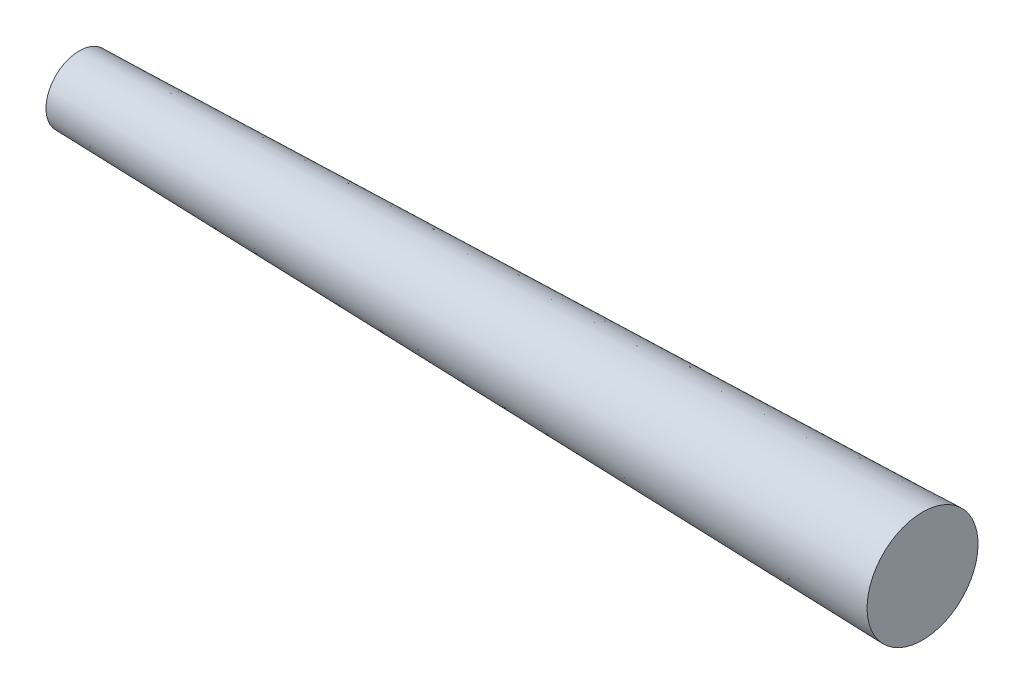
ISO-10303-21;
HEADER;
FILE_DESCRIPTION(('STEP AP214'),'2;1');
FILE_NAME('part.step','',(''),(''),'','','');
FILE_SCHEMA(('AUTOMOTIVE_DESIGN { 1 0 10303 214 1 1 1 1 }'));
ENDSEC;
DATA;
#1=APPLICATION_CONTEXT('core data for automotive mechanical design processes');
#2=APPLICATION_PROTOCOL_DEFINITION('international standard','automotive_design',2000,#1);
#3=PRODUCT_CONTEXT('',#1,'mechanical');
#4=PRODUCT('Part','Part','',(#3));
#5=PRODUCT_RELATED_PRODUCT_CATEGORY('part','',(#4));
#6=PRODUCT_DEFINITION_FORMATION('','',#4);
#7=PRODUCT_DEFINITION_CONTEXT('part definition',#1,'design');
#8=PRODUCT_DEFINITION('design','',#6,#7);
#9=PRODUCT_DEFINITION_SHAPE('','',#8);
#10=(LENGTH_UNIT() NAMED_UNIT(*) SI_UNIT(.MILLI.,.METRE.));
#11=(NAMED_UNIT(*) PLANE_ANGLE_UNIT() SI_UNIT($,.RADIAN.));
#12=(NAMED_UNIT(*) SI_UNIT($,.STERADIAN.) SOLID_ANGLE_UNIT());
#13=UNCERTAINTY_MEASURE_WITH_UNIT(LENGTH_MEASURE(1.E-05),#10,'distance_accuracy_value','');
#14=(GEOMETRIC_REPRESENTATION_CONTEXT(3) GLOBAL_UNCERTAINTY_ASSIGNED_CONTEXT((#13)) GLOBAL_UNIT_ASSIGNED_CONTEXT((#10,
#11,#12)) REPRESENTATION_CONTEXT('',''));
#15=CARTESIAN_POINT('',(0.,0.,0.));
#16=DIRECTION('',(0.,0.,1.));
#17=DIRECTION('',(1.,0.,0.));
#18=AXIS2_PLACEMENT_3D('',#15,#16,#17);
#19=CARTESIAN_POINT('',(0.,2.5,0.));
#20=DIRECTION('',(1.,0.,0.));
#21=DIRECTION('',(0.,1.,0.));
#22=AXIS2_PLACEMENT_3D('',#19,#20,#21);
#23=PLANE('',#22);
#24=CARTESIAN_POINT('',(0.,0.,0.));
#25=DIRECTION('',(1.,0.,0.));
#26=DIRECTION('',(0.,1.,0.));
#27=AXIS2_PLACEMENT_3D('',#24,#25,#26);
#28=CIRCLE('',#27,2.5);
#29=CARTESIAN_POINT('',(0.,2.5,0.));
#30=VERTEX_POINT('',#29);
#31=EDGE_CURVE('E43',#30,#30,#28,.T.);
#32=ORIENTED_EDGE('',*,*,#31,.T.);
#33=EDGE_LOOP('',(#32));
#34=FACE_BOUND('',#33,.T.);
#35=ADVANCED_FACE('F40',(#34),#23,.T.);
#36=CARTESIAN_POINT('',(-38.,0.,0.));
#37=DIRECTION('',(-1.,0.,0.));
#38=DIRECTION('',(0.,-1.,0.));
#39=AXIS2_PLACEMENT_3D('',#36,#37,#38);
#40=PLANE('',#39);
#41=CARTESIAN_POINT('',(-38.,0.,0.));
#42=DIRECTION('',(1.,0.,0.));
#43=DIRECTION('',(0.,1.,0.));
#44=AXIS2_PLACEMENT_3D('',#41,#42,#43);
#45=CIRCLE('',#44,1.5);
#46=CARTESIAN_POINT('',(-38.,1.5,0.));
#47=VERTEX_POINT('',#46);
#48=EDGE_CURVE('E10',#47,#47,#45,.T.);
#49=ORIENTED_EDGE('',*,*,#48,.F.);
#50=EDGE_LOOP('',(#49));
#51=FACE_BOUND('',#50,.T.);
#52=ADVANCED_FACE('F55',(#51),#40,.T.);
#53=CARTESIAN_POINT('',(0.,0.,0.));
#54=DIRECTION('',(1.,0.,0.));
#55=DIRECTION('',(0.,1.,0.));
#56=AXIS2_PLACEMENT_3D('',#53,#54,#55);
#57=CONICAL_SURFACE('',#56,2.5,0.0263097172529222);
#58=ORIENTED_EDGE('',*,*,#48,.T.);
#59=EDGE_LOOP('',(#58));
#60=FACE_BOUND('',#59,.T.);
#61=ORIENTED_EDGE('',*,*,#31,.F.);
#62=EDGE_LOOP('',(#61));
#63=FACE_BOUND('',#62,.T.);
#64=ADVANCED_FACE('F49',(#60,#63),#57,.T.);
#65=CLOSED_SHELL('',(#35,#52,#64));
#66=MANIFOLD_SOLID_BREP('B2',#65);
#67=ADVANCED_BREP_SHAPE_REPRESENTATION('',(#18,#66),#14);
#68=SHAPE_DEFINITION_REPRESENTATION(#9,#67);
ENDSEC;
END-ISO-10303-21;
